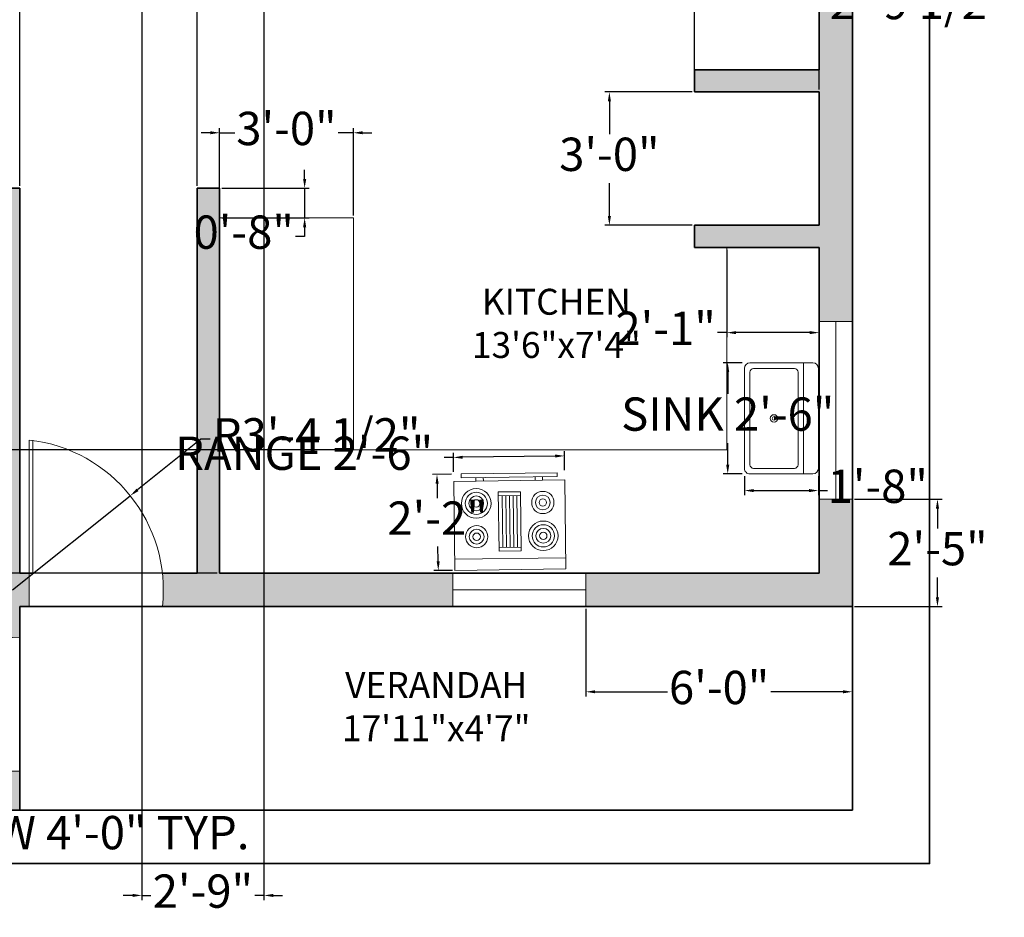
# Model space of a CAD drawing. Units: inches. Extents: x 1649 to 2193, y 1782 to 2280.
# Tile 2 of 3: x 1905 to 2171, y 1782 to 2024. Entities that reach past the tile are written whole.
import ezdxf

# ---------------------------------------------------------------- set-up
doc = ezdxf.new("R2010")
doc.units = ezdxf.units.IN
for name, color, linetype, lineweight in [('A-ANNO-DIMS', 2, 'Continuous', 18), ('A-ANNO-TTLB', 7, 'Continuous', 35), ('A-AREA-IDEN', 7, 'Continuous', 25), ('A-DOOR', 3, 'Continuous', 18), ('A-EQPM', 8, 'Continuous', 18), ('A-FLOR-CASE', 8, 'Continuous', 20), ('A-FLOR-FIXT', 9, 'Continuous', 18), ('A-GLAZ', 4, 'Continuous', 18), ('A-WALL', 7, 'Continuous', 35)]:
    doc.layers.add(name, color=color, linetype=linetype, lineweight=lineweight)
doc.layers.add('A-WALL-PATT', color=18, linetype='Continuous', lineweight=13, true_color=0x000000)
doc.styles.get("Standard").update_dxf_attribs({"font": 'arial.ttf'})
doc.dimstyles.new('ISO-25', dxfattribs={"dimtxt": 9, "dimasz": 2.5, "dimexe": 1.25, "dimexo": 0.625, "dimgap": 2, "dimtad": 0, "dimtih": 1, "dimtoh": 1, "dimdec": 1, "dimlunit": 4, "dimtxsty": 'Standard', "dimcen": 2.5, "dimadec": 0, "dimazin": 0, "dimtfac": 0.5, "dimtdec": 1, "dimtmove": 0, "dimatfit": 3, "dimfxl": 1, "dimarcsym": 0})

# ---------------------------------------------------------------- blocks, each defined once
blk = doc.blocks.new('Range-Oven - 30 in top')
for p, q in [((0, -3), (30, -3)), ((12, -6), (18, -6)), ((13, -20), (13, -6)), ((14, -6), (14, -20)), ((15, -20), (15, -6)), ((16, -6), (16, -20)), ((17, -20), (17, -6)), ((18, -20), (12, -20)), ((6, -24), (6, -25)), ((8, -25), (8, -24)), ((22, -25), (22, -24)), ((24, -24), (24, -25))]:
    blk.add_line(p, q)
for points in [[(0, -24), (0, 0), (30, 0), (30, -24)], [(12, -21), (12, -5), (18, -5), (18, -21)], [(2, -26), (2, -25), (28, -25), (28, -26)]]:
    blk.add_lwpolyline(points, close=True)
for centre, radius in [((6, -9), 4), ((6, -9), 3), ((6, -9), 2), ((24, -9), 3), ((24, -9), 2), ((6, -9), 1), ((24, -9), 1), ((6, -18), 3), ((24, -18), 4), ((24, -18), 3), ((6, -18), 2), ((6, -18), 1), ((24, -18), 2), ((24, -18), 1)]:
    blk.add_circle(centre, radius)
blk = doc.blocks.new('Sink-single - 30 in top')
blk.add_line((-15, -3.999996), (15, -3.999996))
for points in [[(-13.5, 0), (13.5, 0)], [(-15, -18.499996), (-15, -1.5)], [(15, -1.5), (15, -18.499996)], [(-13.5, -17.499996), (-13.5, -6.499996)], [(-12.5, -5.499996), (12.5, -5.499996)], [(13.5, -6.499996), (13.5, -17.499996)], [(12.5, -18.499996), (-12.5, -18.499996)], [(13.5, -19.999996), (-13.5, -19.999996)]]:
    blk.add_lwpolyline(points)
for radius in [1, 0.5]:
    blk.add_circle((0, -11.999996), radius)
for centre, radius, start, end in [((-13.5, -1.5), 1.5, 90, 180), ((13.5, -1.5), 1.5, 0, 90), ((-12.5, -6.499996), 1, 90, 180), ((12.5, -6.499996), 1, 0, 90), ((-13.5, -18.499996), 1.5, 180, 270), ((-12.5, -17.499996), 1, 180, 270), ((12.5, -17.499996), 1, 270, 0), ((13.5, -18.499996), 1.5, 270, 0)]:
    blk.add_arc(centre, radius, start, end)
blk = doc.blocks.new('DOOR-36IN')
for p, q in [((0, 6), (0, 42)), ((1, 6), (1, 42)), ((0, 6), (0, 0))]:
    blk.add_line(p, q)
blk.add_arc((-3, 3), 39.12, 355.6013, 85.6013)
blk = doc.blocks.new('WIN-48IN')
for p, q in [((0, 48), (9, 48)), ((4.5, 48), (4.5, 0)), ((0, 0), (9, 0))]:
    blk.add_line(p, q)
blk = doc.blocks.new('WIN-36IN')
for p, q in [((0, 9), (0, 0)), ((36, 9), (36, 0)), ((0, 4.5), (36, 4.5))]:
    blk.add_line(p, q)
blk = doc.blocks.new('*D23')
at = {"layer": 'A-ANNO-DIMS', "color": 0, "lineweight": -2, "transparency": 16777216}
for p, q in [((1803.13, 1810.03), (1803.13, 1802.2)), ((1851.13, 1810.03), (1851.13, 1802.2)), ((1805.63, 1803.45), (1848.63, 1803.45)), ((1851.13, 1803.45), (1853.63, 1803.45))]:
    blk.add_line(p, q, dxfattribs=at)
at = {"layer": 'A-ANNO-DIMS', "color": 0, "transparency": 16777216}
for points in [[(1805.63, 1803.87), (1805.63, 1803.04), (1803.13, 1803.45)], [(1848.63, 1803.87), (1848.63, 1803.04), (1851.13, 1803.45)]]:
    blk.add_solid(points, dxfattribs=at)
at = {"layer": 'Defpoints', "color": 0, "transparency": 16777216}
for p in [(1803.13, 1810.65), (1851.13, 1810.65), (1851.13, 1803.45)]:
    blk.add_point(p, dxfattribs=at)
at = {"layer": 'A-ANNO-DIMS', "color": 0, "transparency": 16777216, "insert": (1912.57, 1803.45), "char_height": 9, "attachment_point": 5}
blk.add_mtext('WINDOW 4\'-0" TYP.', dxfattribs=at)
blk = doc.blocks.new('*D29')
at = {"layer": 'A-ANNO-DIMS', "color": 0, "lineweight": -2, "transparency": 16777216}
for p, q in [((2022.33, 1905.95), (2019.83, 1905.92)), ((2022.39, 1902.08), (2022.32, 1907.2)), ((2049.83, 1906.32), (2024.83, 1905.98)), ((2052.38, 1902.48), (2052.31, 1907.61))]:
    blk.add_line(p, q, dxfattribs=at)
at = {"layer": 'A-ANNO-DIMS', "color": 0, "transparency": 16777216}
for points in [[(2024.83, 1906.4), (2024.84, 1905.57), (2022.33, 1905.95)], [(2049.82, 1906.74), (2049.84, 1905.91), (2052.33, 1906.36)]]:
    blk.add_solid(points, dxfattribs=at)
at = {"layer": 'Defpoints', "color": 0, "transparency": 16777216}
for p in [(2022.33, 1905.95), (2022.39, 1901.45), (2052.39, 1901.86)]:
    blk.add_point(p, dxfattribs=at)
at = {"layer": 'A-ANNO-DIMS', "color": 0, "transparency": 16777216, "insert": (1982, 1905.92), "char_height": 9, "attachment_point": 5}
blk.add_mtext('RANGE 2\'-6"', dxfattribs=at)
blk = doc.blocks.new('*D30')
at = {"layer": 'A-ANNO-DIMS', "color": 0, "lineweight": -2, "transparency": 16777216}
for p, q in [((2021.77, 1901.44), (2016.64, 1901.37)), ((2017.93, 1898.89), (2017.98, 1894.91)), ((2018.21, 1877.89), (2018.16, 1881.87)), ((2022.12, 1875.44), (2017, 1875.38))]:
    blk.add_line(p, q, dxfattribs=at)
at = {"layer": 'A-ANNO-DIMS', "color": 0, "transparency": 16777216}
for points in [[(2018.34, 1898.9), (2017.51, 1898.88), (2017.89, 1901.39)], [(2018.63, 1877.9), (2017.8, 1877.89), (2018.25, 1875.39)]]:
    blk.add_solid(points, dxfattribs=at)
at = {"layer": 'Defpoints', "color": 0, "transparency": 16777216}
for p in [(2022.39, 1901.45), (2018.25, 1875.39), (2022.75, 1875.45)]:
    blk.add_point(p, dxfattribs=at)
at = {"layer": 'A-ANNO-DIMS', "color": 0, "transparency": 16777216, "insert": (2018.07, 1888.39), "char_height": 9, "attachment_point": 5}
blk.add_mtext('2\'-2"', dxfattribs=at)
blk = doc.blocks.new('*D31')
at = {"layer": 'A-ANNO-DIMS', "color": 0, "lineweight": -2, "transparency": 16777216}
for p, q in [((2100.33, 1931.49), (2095.21, 1931.49)), ((2096.46, 1928.99), (2096.46, 1923.15)), ((2096.46, 1903.99), (2096.46, 1909.84)), ((2100.33, 1901.49), (2095.21, 1901.49))]:
    blk.add_line(p, q, dxfattribs=at)
at = {"layer": 'A-ANNO-DIMS', "color": 0, "transparency": 16777216}
for points in [[(2096.04, 1928.99), (2096.87, 1928.99), (2096.46, 1931.49)], [(2096.04, 1903.99), (2096.87, 1903.99), (2096.46, 1901.49)]]:
    blk.add_solid(points, dxfattribs=at)
at = {"layer": 'Defpoints', "color": 0, "transparency": 16777216}
for p in [(2100.96, 1931.49), (2096.46, 1901.49), (2100.96, 1901.49)]:
    blk.add_point(p, dxfattribs=at)
at = {"layer": 'A-ANNO-DIMS', "color": 0, "transparency": 16777216, "insert": (2096.46, 1916.49), "char_height": 9, "attachment_point": 5}
blk.add_mtext('SINK 2\'-6"', dxfattribs=at)
blk = doc.blocks.new('*D32')
at = {"layer": 'A-ANNO-DIMS', "color": 0, "lineweight": -2, "transparency": 16777216}
for p, q in [((2100.96, 1900.87), (2100.96, 1895.74)), ((2120.96, 1900.87), (2120.96, 1895.74)), ((2103.46, 1896.99), (2118.46, 1896.99)), ((2120.96, 1896.99), (2123.46, 1896.99))]:
    blk.add_line(p, q, dxfattribs=at)
at = {"layer": 'A-ANNO-DIMS', "color": 0, "transparency": 16777216}
for points in [[(2103.46, 1897.41), (2103.46, 1896.58), (2100.96, 1896.99)], [(2118.46, 1897.41), (2118.46, 1896.58), (2120.96, 1896.99)]]:
    blk.add_solid(points, dxfattribs=at)
at = {"layer": 'Defpoints', "color": 0, "transparency": 16777216}
for p in [(2100.96, 1901.49), (2120.96, 1901.49), (2120.96, 1896.99)]:
    blk.add_point(p, dxfattribs=at)
at = {"layer": 'A-ANNO-DIMS', "color": 0, "transparency": 16777216, "insert": (2137, 1896.99), "char_height": 9, "attachment_point": 5}
blk.add_mtext('1\'-8"', dxfattribs=at)
blk = doc.blocks.new('*D36')
at = {"layer": 'A-ANNO-DIMS', "color": 0, "lineweight": -2, "transparency": 16777216}
for p, q in [((1905.13, 1979.28), (1905.13, 2266.9)), ((1953.13, 1979.28), (1953.13, 2266.9)), ((1907.63, 2265.65), (1914.99, 2265.65)), ((1950.63, 2265.65), (1943.27, 2265.65))]:
    blk.add_line(p, q, dxfattribs=at)
at = {"layer": 'A-ANNO-DIMS', "color": 0, "transparency": 16777216}
for points in [[(1907.63, 2266.07), (1907.63, 2265.24), (1905.13, 2265.65)], [(1950.63, 2266.07), (1950.63, 2265.24), (1953.13, 2265.65)]]:
    blk.add_solid(points, dxfattribs=at)
at = {"layer": 'Defpoints', "color": 0, "transparency": 16777216}
for p in [(1953.13, 2265.65), (1905.13, 1978.65), (1953.13, 1978.65)]:
    blk.add_point(p, dxfattribs=at)
at = {"layer": 'A-ANNO-DIMS', "color": 0, "transparency": 16777216, "insert": (1929.13, 2265.65), "char_height": 9, "attachment_point": 5}
blk.add_mtext('4\'-0"', dxfattribs=at)
blk = doc.blocks.new('*D41')
at = {"layer": 'A-ANNO-DIMS', "color": 0, "lineweight": -2, "transparency": 16777216}
for p, q in [((2058.13, 1865.03), (2058.13, 1841.4)), ((2130.13, 1865.03), (2130.13, 1841.4)), ((2060.63, 1842.65), (2080.14, 1842.65)), ((2127.63, 1842.65), (2108.12, 1842.65))]:
    blk.add_line(p, q, dxfattribs=at)
at = {"layer": 'A-ANNO-DIMS', "color": 0, "transparency": 16777216}
for points in [[(2060.63, 1843.07), (2060.63, 1842.24), (2058.13, 1842.65)], [(2127.63, 1843.07), (2127.63, 1842.24), (2130.13, 1842.65)]]:
    blk.add_solid(points, dxfattribs=at)
at = {"layer": 'Defpoints', "color": 0, "transparency": 16777216}
for p in [(2058.13, 1865.65), (2130.13, 1865.65), (2058.13, 1842.65)]:
    blk.add_point(p, dxfattribs=at)
at = {"layer": 'A-ANNO-DIMS', "color": 0, "transparency": 16777216, "insert": (2094.13, 1842.65), "char_height": 9, "attachment_point": 5}
blk.add_mtext('6\'-0"', dxfattribs=at)
blk = doc.blocks.new('*D42')
at = {"layer": 'A-ANNO-DIMS', "color": 0, "lineweight": -2, "transparency": 16777216}
for p, q in [((2130.75, 1894.65), (2154.38, 1894.65)), ((2153.13, 1892.15), (2153.13, 1886.75)), ((2153.13, 1868.15), (2153.13, 1873.56)), ((2130.75, 1865.65), (2154.38, 1865.65))]:
    blk.add_line(p, q, dxfattribs=at)
at = {"layer": 'A-ANNO-DIMS', "color": 0, "transparency": 16777216}
for points in [[(2152.71, 1892.15), (2153.55, 1892.15), (2153.13, 1894.65)], [(2152.71, 1868.15), (2153.55, 1868.15), (2153.13, 1865.65)]]:
    blk.add_solid(points, dxfattribs=at)
at = {"layer": 'Defpoints', "color": 0, "transparency": 16777216}
for p in [(2130.13, 1894.65), (2153.13, 1894.65), (2130.13, 1865.65)]:
    blk.add_point(p, dxfattribs=at)
at = {"layer": 'A-ANNO-DIMS', "color": 0, "transparency": 16777216, "insert": (2153.13, 1880.15), "char_height": 9, "attachment_point": 5}
blk.add_mtext('2\'-5"', dxfattribs=at)
blk = doc.blocks.new('*D51')
at = {"layer": 'A-ANNO-DIMS', "color": 0, "lineweight": -2, "transparency": 16777216}
for p, q in [((1938.13, 2212.02), (1938.13, 1786.4)), ((1971.13, 2201.52), (1971.13, 1786.4)), ((1935.63, 1787.65), (1933.13, 1787.65)), ((1938.13, 1787.65), (1940.59, 1787.65)), ((1971.13, 1787.65), (1968.67, 1787.65)), ((1973.63, 1787.65), (1976.13, 1787.65))]:
    blk.add_line(p, q, dxfattribs=at)
at = {"layer": 'A-ANNO-DIMS', "color": 0, "transparency": 16777216}
for points in [[(1935.63, 1788.07), (1935.63, 1787.24), (1938.13, 1787.65)], [(1973.63, 1788.07), (1973.63, 1787.24), (1971.13, 1787.65)]]:
    blk.add_solid(points, dxfattribs=at)
at = {"layer": 'Defpoints', "color": 0, "transparency": 16777216}
for p in [(1938.13, 2212.65), (1971.13, 2202.15), (1971.13, 1787.65)]:
    blk.add_point(p, dxfattribs=at)
at = {"layer": 'A-ANNO-DIMS', "color": 0, "transparency": 16777216, "insert": (1954.63, 1787.65), "char_height": 9, "attachment_point": 5}
blk.add_mtext('2\'-9"', dxfattribs=at)
blk = doc.blocks.new('*D54')
at = {"layer": 'A-ANNO-DIMS', "color": 0, "lineweight": -2, "transparency": 16777216}
for p, q in [((2087.48, 2005.28), (2087.48, 2028.9)), ((2089.98, 2027.65), (2118.63, 2027.65)), ((2121.13, 2005.28), (2121.13, 2028.9)), ((2121.13, 2027.65), (2123.63, 2027.65))]:
    blk.add_line(p, q, dxfattribs=at)
at = {"layer": 'A-ANNO-DIMS', "color": 0, "transparency": 16777216}
for points in [[(2089.98, 2028.07), (2089.98, 2027.24), (2087.48, 2027.65)], [(2118.63, 2028.07), (2118.63, 2027.24), (2121.13, 2027.65)]]:
    blk.add_solid(points, dxfattribs=at)
at = {"layer": 'Defpoints', "color": 0, "transparency": 16777216}
for p in [(2121.13, 2027.65), (2087.48, 2004.65), (2121.13, 2004.65)]:
    blk.add_point(p, dxfattribs=at)
at = {"layer": 'A-ANNO-DIMS', "color": 0, "transparency": 16777216, "insert": (2148.15, 2027.65), "char_height": 9, "attachment_point": 5}
blk.add_mtext('2\'-9 1/2"', dxfattribs=at)
blk = doc.blocks.new('*D55')
at = {"layer": 'A-ANNO-DIMS', "color": 0, "lineweight": -2, "transparency": 16777216}
for p, q in [((2086.85, 2004.65), (2063.23, 2004.65)), ((2064.48, 2002.15), (2064.48, 1993.25)), ((2064.48, 1971.15), (2064.48, 1980.05)), ((2086.85, 1968.65), (2063.23, 1968.65))]:
    blk.add_line(p, q, dxfattribs=at)
at = {"layer": 'A-ANNO-DIMS', "color": 0, "transparency": 16777216}
for points in [[(2064.06, 2002.15), (2064.89, 2002.15), (2064.48, 2004.65)], [(2064.06, 1971.15), (2064.89, 1971.15), (2064.48, 1968.65)]]:
    blk.add_solid(points, dxfattribs=at)
at = {"layer": 'Defpoints', "color": 0, "transparency": 16777216}
for p in [(2064.48, 2004.65), (2087.48, 2004.65), (2087.48, 1968.65)]:
    blk.add_point(p, dxfattribs=at)
at = {"layer": 'A-ANNO-DIMS', "color": 0, "transparency": 16777216, "insert": (2064.48, 1986.65), "char_height": 9, "attachment_point": 5}
blk.add_mtext('3\'-0"', dxfattribs=at)
blk = doc.blocks.new('*D56')
at = {"layer": 'A-ANNO-DIMS', "color": 0, "lineweight": -2, "transparency": 16777216}
for p, q in [((2096.22, 1962.03), (2096.22, 1938.4)), ((2121.13, 1962.03), (2121.13, 1938.4)), ((2096.22, 1939.65), (2093.72, 1939.65)), ((2118.63, 1939.65), (2098.72, 1939.65))]:
    blk.add_line(p, q, dxfattribs=at)
at = {"layer": 'A-ANNO-DIMS', "color": 0, "transparency": 16777216}
for points in [[(2098.72, 1940.07), (2098.72, 1939.24), (2096.22, 1939.65)], [(2118.63, 1940.07), (2118.63, 1939.24), (2121.13, 1939.65)]]:
    blk.add_solid(points, dxfattribs=at)
at = {"layer": 'Defpoints', "color": 0, "transparency": 16777216}
for p in [(2096.22, 1962.65), (2121.13, 1962.65), (2096.22, 1939.65)]:
    blk.add_point(p, dxfattribs=at)
at = {"layer": 'A-ANNO-DIMS', "color": 0, "transparency": 16777216, "insert": (2079.68, 1939.65), "char_height": 9, "attachment_point": 5}
blk.add_mtext('2\'-1"', dxfattribs=at)
blk = doc.blocks.new('*D57')
at = {"layer": 'A-ANNO-DIMS', "color": 0, "lineweight": -2, "transparency": 16777216}
for p, q in [((1956.63, 1993.63), (1954.13, 1993.63)), ((1959.13, 1971.26), (1959.13, 1994.88)), ((1959.13, 1993.63), (1963.25, 1993.63)), ((1995.3, 1993.63), (1991.17, 1993.63)), ((1995.3, 1971.26), (1995.3, 1994.88)), ((1997.8, 1993.63), (2000.3, 1993.63))]:
    blk.add_line(p, q, dxfattribs=at)
at = {"layer": 'A-ANNO-DIMS', "color": 0, "transparency": 16777216}
for points in [[(1956.63, 1994.05), (1956.63, 1993.22), (1959.13, 1993.63)], [(1997.8, 1994.05), (1997.8, 1993.22), (1995.3, 1993.63)]]:
    blk.add_solid(points, dxfattribs=at)
at = {"layer": 'Defpoints', "color": 0, "transparency": 16777216}
for p in [(1995.3, 1993.63), (1959.13, 1970.63), (1995.3, 1970.63)]:
    blk.add_point(p, dxfattribs=at)
at = {"layer": 'A-ANNO-DIMS', "color": 0, "transparency": 16777216, "insert": (1977.21, 1993.63), "char_height": 9, "attachment_point": 5}
blk.add_mtext('3\'-0"', dxfattribs=at)
blk = doc.blocks.new('*D58')
at = {"layer": 'A-ANNO-DIMS', "color": 0, "lineweight": -2, "transparency": 16777216}
for p, q in [((1994.67, 1908.03), (1671.31, 1908.03)), ((1672.56, 1905.53), (1672.56, 1898)), ((1672.56, 1877.15), (1672.56, 1884.69)), ((1958.5, 1874.65), (1671.31, 1874.65))]:
    blk.add_line(p, q, dxfattribs=at)
at = {"layer": 'A-ANNO-DIMS', "color": 0, "transparency": 16777216}
for points in [[(1672.15, 1905.53), (1672.98, 1905.53), (1672.56, 1908.03)], [(1672.15, 1877.15), (1672.98, 1877.15), (1672.56, 1874.65)]]:
    blk.add_solid(points, dxfattribs=at)
at = {"layer": 'Defpoints', "color": 0, "transparency": 16777216}
for p in [(1995.3, 1908.03), (1672.56, 1874.65), (1959.13, 1874.65)]:
    blk.add_point(p, dxfattribs=at)
at = {"layer": 'A-ANNO-DIMS', "color": 0, "transparency": 16777216, "insert": (1672.56, 1891.34), "char_height": 9, "attachment_point": 5}
blk.add_mtext('2\'-9 1/2"', dxfattribs=at)
blk = doc.blocks.new('*D59')
at = {"layer": 'A-ANNO-DIMS', "color": 0, "lineweight": -2, "transparency": 16777216}
for p, q in [((1982.13, 1981.15), (1982.13, 1983.65)), ((1959.75, 1978.65), (1983.38, 1978.65)), ((1982.13, 1978.65), (1982.13, 1970.63)), ((1959.75, 1970.63), (1983.38, 1970.63)), ((1982.13, 1968.13), (1982.13, 1965.63)), ((1982.13, 1965.63), (1979.63, 1965.63))]:
    blk.add_line(p, q, dxfattribs=at)
at = {"layer": 'A-ANNO-DIMS', "color": 0, "transparency": 16777216}
for points in [[(1981.71, 1981.15), (1982.55, 1981.15), (1982.13, 1978.65)], [(1981.71, 1968.13), (1982.55, 1968.13), (1982.13, 1970.63)]]:
    blk.add_solid(points, dxfattribs=at)
at = {"layer": 'Defpoints', "color": 0, "transparency": 16777216}
for p in [(1959.13, 1978.65), (1959.13, 1970.63), (1982.13, 1970.63)]:
    blk.add_point(p, dxfattribs=at)
at = {"layer": 'A-ANNO-DIMS', "color": 0, "transparency": 16777216, "insert": (1965.67, 1965.63), "char_height": 9, "attachment_point": 5}
blk.add_mtext('0\'-8"', dxfattribs=at)
blk = doc.blocks.new('*D61')
at = {"layer": 'A-ANNO-DIMS', "color": 0, "lineweight": -2, "transparency": 16777216}
for p, q in [((1954.1, 1910.88), (1936.96, 1897.17)), ((1956.6, 1910.88), (1954.1, 1910.88)), ((1903.19, 1870.15), (1935.01, 1895.61))]:
    blk.add_line(p, q, dxfattribs=at)
at = {"layer": 'A-ANNO-DIMS', "color": 0, "transparency": 16777216}
blk.add_solid([(1936.7, 1897.5), (1937.22, 1896.84), (1935.01, 1895.61)], dxfattribs=at)
at = {"layer": 'Defpoints', "color": 0, "transparency": 16777216}
for p in [(1935.01, 1895.61), (1903.19, 1870.15)]:
    blk.add_point(p, dxfattribs=at)
at = {"layer": 'A-ANNO-DIMS', "color": 0, "transparency": 16777216, "insert": (1985.35, 1910.88), "char_height": 9, "attachment_point": 5}
blk.add_mtext('R3\'-4 1/2"', dxfattribs=at)

msp = doc.modelspace()

# ---------------------------------------------------------------- hatches: boundary and pattern name
at = {"layer": 'A-WALL-PATT'}
h = msp.add_hatch(color=256, dxfattribs=at)
h.dxf.hatch_style = 1
h.paths.add_polyline_path([(1926.13, 2242.65), (1746.13, 2242.65), (1746.13, 2203.65), (1755.13, 2203.65), (1755.13, 2233.65), (1899.13, 2233.65), (1899.13, 2113.65), (1897.63, 2113.65), (1897.63, 2107.65), (1899.13, 2107.65), (1907.03, 2107.65), (1907.03, 2113.65), (1905.13, 2113.65), (1905.13, 2233.65), (1926.13, 2233.65)])
h.paths.add_polyline_path([(2130.13, 2242.65), (1950.13, 2242.65), (1950.13, 2233.65), (1971.13, 2233.65), (1971.13, 2113.65), (1937.03, 2113.65, -0.045361), (1937.03, 2107.65), (1978.81, 2107.65), (1978.81, 2113.65), (1977.13, 2113.65), (1977.13, 2233.65), (2121.13, 2233.65), (2121.13, 2203.65), (2130.13, 2203.65)])
h.paths.add_polyline_path([(2130.13, 2143.65), (2121.13, 2143.65), (2121.13, 2113.65), (2014.81, 2113.65, -0.038405), (2014.81, 2107.65), (2121.13, 2107.65), (2121.13, 2089.15), (2130.13, 2089.15)])
h.paths.add_polyline_path([(1824.23, 2113.65), (1755.13, 2113.65), (1755.13, 2143.65), (1746.13, 2143.65), (1746.13, 2093.65), (1755.13, 2093.65), (1755.13, 2107.65), (1824.23, 2107.65, -0.045361)])
h.paths.add_polyline_path([(1862.13, 2055.65), (1862.13, 2107.65), (1863.33, 2107.65, -0.038218), (1863.33, 2113.65), (1854.23, 2113.65), (1854.23, 2107.65), (1856.13, 2107.65), (1856.13, 2055.65), (1755.13, 2055.65), (1755.13, 2069.65), (1746.13, 2069.65), (1746.13, 2032.15), (1755.13, 2032.15), (1755.13, 2049.65), (1862.13, 2049.65)])
h.paths.add_polyline_path([(2130.13, 2029.15), (2121.13, 2029.15), (2121.13, 2010.65), (2087.48, 2010.65), (2087.48, 2004.65), (2121.13, 2004.65), (2121.13, 1968.65), (2087.48, 1968.65), (2087.48, 1962.65), (2121.13, 1962.65), (2121.13, 1942.65), (2130.13, 1942.65)])
h.paths.add_polyline_path([(2022.13, 1874.65), (1959.13, 1874.65), (1959.13, 1978.65), (1953.13, 1978.65), (1953.13, 1874.65), (1943.69, 1874.65, -0.055385), (1943.69, 1865.65), (2022.13, 1865.65)])
h.paths.add_polyline_path([(2130.13, 1894.65), (2121.13, 1894.65), (2121.13, 1874.65), (2058.13, 1874.65), (2058.13, 1865.65), (2121.13, 1865.65), (2130.13, 1865.65)])
h.paths.add_polyline_path([(1755.13, 1972.65), (1859.98, 1972.65, -0.038405), (1859.98, 1978.65), (1755.13, 1978.65), (1755.13, 1996.15), (1746.13, 1996.15), (1746.13, 1920.15), (1755.13, 1920.15)])
h.paths.add_polyline_path([(1803.13, 1819.65), (1755.13, 1819.65), (1755.13, 1872.15), (1746.13, 1872.15), (1746.13, 1810.65), (1803.13, 1810.65)])
h.paths.add_polyline_path([(1905.13, 1819.65), (1905.13, 1821.19), (1899.13, 1821.19), (1899.13, 1819.65), (1851.13, 1819.65), (1851.13, 1810.65), (1905.13, 1810.65)])
h.paths.add_polyline_path([(1907.69, 1874.65), (1905.13, 1874.65), (1905.13, 1972.65), (1905.13, 1978.65), (1895.98, 1978.65), (1895.98, 1972.65), (1899.13, 1972.65), (1899.13, 1857.19, -0.038405), (1905.13, 1857.19), (1905.13, 1865.65), (1907.69, 1865.65)])

# ---------------------------------------------------------------- linework, layer by layer
at = {"layer": 'A-ANNO-TTLB'}
msp.add_lwpolyline([(1708.93, 2280.02), (2150.99, 2280.02), (2150.99, 1796.25), (1708.93, 1796.25)], close=True, dxfattribs=at)
at = {"layer": 'A-DOOR'}
for p, q in [((1907.69, 1874.65), (1907.69, 1910.65)), ((1908.69, 1874.65), (1908.69, 1910.65)), ((1907.69, 1874.65), (1907.69, 1865.65))]:
    msp.add_line(p, q, dxfattribs=at)
msp.add_arc((1903.19, 1870.15), 40.75, 353.6598, 83.6598, dxfattribs=at)
at = {"layer": 'A-FLOR-CASE'}
for p, q in [((1995.3, 1970.63), (1959.13, 1970.63)), ((1995.3, 1908.03), (1995.3, 1970.63)), ((2096.22, 1962.65), (2096.22, 1908.03)), ((2096.22, 1908.03), (1995.3, 1908.03))]:
    msp.add_line(p, q, dxfattribs=at)
at = {"layer": 'A-WALL'}
for p, q in [((2130.13, 2242.65), (2130.13, 1810.65)), ((2121.13, 2107.65), (2121.13, 2010.65)), ((2121.13, 2010.65), (2087.48, 2010.65)), ((2087.48, 2004.65), (2087.48, 2010.65)), ((2121.13, 2004.65), (2087.48, 2004.65)), ((2121.13, 1968.65), (2121.13, 2004.65)), ((2121.13, 2004.65), (2121.13, 1968.65)), ((1905.13, 1978.65), (1755.13, 1978.65)), ((1905.13, 1972.65), (1905.13, 1978.65)), ((1953.13, 1978.65), (1953.13, 1874.65)), ((1953.13, 1978.65), (1959.13, 1978.65)), ((1959.13, 1978.65), (1959.13, 1874.65)), ((1905.13, 1874.65), (1905.13, 1972.65)), ((2121.13, 1968.65), (2087.48, 1968.65)), ((2087.48, 1968.65), (2087.48, 1962.65)), ((2121.13, 1962.65), (2087.48, 1962.65)), ((2121.13, 1962.65), (2121.13, 1874.65)), ((1908.69, 1874.65), (1905.13, 1874.65)), ((1953.13, 1874.65), (1943.69, 1874.65)), ((2121.13, 1874.65), (1959.13, 1874.65)), ((1905.13, 1819.65), (1905.13, 1865.65)), ((2121.13, 1865.65), (1905.13, 1865.65)), ((2121.13, 1865.65), (2130.13, 1865.65)), ((1905.13, 1819.65), (1905.13, 1810.65)), ((2130.13, 1810.65), (1746.13, 1810.65))]:
    msp.add_line(p, q, dxfattribs=at)

# ---------------------------------------------------------------- block references
at = {"layer": 'A-DOOR', "rotation": 89.99999999999905}
msp.add_blockref('DOOR-36IN', (1905.13, 1821.19), dxfattribs=at)
at = {"layer": 'A-EQPM', "rotation": 180.7771274632593}
msp.add_blockref('Range-Oven - 30 in top', (2052.74, 1875.86), dxfattribs=at)
at = {"layer": 'A-FLOR-FIXT', "rotation": 270}
msp.add_blockref('Sink-single - 30 in top', (2120.96, 1916.49), dxfattribs=at)
at = {"layer": 'A-GLAZ'}
for name, p in [('WIN-48IN', (2121.13, 1894.65)), ('WIN-36IN', (2022.13, 1865.65))]:
    msp.add_blockref(name, p, dxfattribs=at)

# ---------------------------------------------------------------- texts
at = {"layer": 'A-AREA-IDEN', "char_height": 7, "attachment_point": 1}
for s, width, insert in [('\\pxqc;{\\fArial|b1|i0|c0|p34;KITCHEN\\P13\'6"x7\'4"}', 92.1713, (2004.05, 1951.49)), ('\\pxqc;{\\fArial|b1|i0|c0|p34;VERANDAH\\P17\'11"x4\'7"}', 107.1133, (1964.13, 1847.98))]:
    msp.add_mtext_dynamic_manual_height_columns(s, width=width, gutter_width=12.5, heights=[0], dxfattribs=dict(at, insert=insert))

# ---------------------------------------------------------------- dimensions: what is measured, and where the dimension line sits
at = {"layer": 'A-ANNO-DIMS'}
for base, p1, p2, picture, middle in [((1953.13, 2265.65), (1905.13, 1978.65), (1953.13, 1978.65), '*D36', (1929.13, 2265.65)), ((1971.13, 1787.65), (1938.13, 2212.65), (1971.13, 2202.15), '*D51', (1954.63, 1787.65)), ((2121.1289, 2027.6524), (2087.4781, 2004.6524), (2121.1289, 2004.6524), '*D54', (2148.1535, 2027.6524)), ((1995.3, 1993.63), (1959.13, 1970.63), (1995.3, 1970.63), '*D57', (1977.21, 1993.63)), ((2120.96, 1896.99), (2100.96, 1901.49), (2120.96, 1901.49), '*D32', (2137, 1896.99))]:
    dim = msp.add_linear_dim(base=base, p1=p1, p2=p2, dimstyle='ISO-25', override={"dimdec": 1, "dimlfac": 1, "dimrnd": 0, "dimzin": 1, "dimdsep": 46, "dimlunit": 4, "dimfrac": 2}, dxfattribs=at)
    dim.commit()
    dim.dimension.update_dxf_attribs({"geometry": picture, "text_midpoint": middle})
for base, p1, p2, angle, picture, middle in [((2064.48, 2004.65), (2087.48, 1968.65), (2087.48, 2004.65), 90, '*D55', (2064.48, 1986.65)), ((1982.13, 1970.63), (1959.13, 1978.65), (1959.13, 1970.63), 270, '*D59', (1965.67, 1965.63)), ((2096.22, 1939.65), (2121.13, 1962.65), (2096.22, 1962.65), 180, '*D56', (2079.68, 1939.65)), ((1672.56, 1874.65), (1995.3, 1908.03), (1959.13, 1874.65), 90, '*D58', (1672.56, 1891.34)), ((2018.25, 1875.39), (2022.39, 1901.45), (2022.75, 1875.45), 270.7771, '*D30', (2018.07, 1888.39)), ((2153.13, 1894.65), (2130.13, 1865.65), (2130.13, 1894.65), 90, '*D42', (2153.13, 1880.15)), ((2058.13, 1842.65), (2130.13, 1865.65), (2058.13, 1865.65), 180, '*D41', (2094.13, 1842.65))]:
    dim = msp.add_linear_dim(base=base, p1=p1, p2=p2, angle=angle, dimstyle='ISO-25', override={"dimdec": 1, "dimlfac": 1, "dimrnd": 0, "dimzin": 1, "dimdsep": 46, "dimlunit": 4, "dimfrac": 2}, dxfattribs=at)
    dim.commit()
    dim.dimension.update_dxf_attribs({"geometry": picture, "text_midpoint": middle})
for base, p1, p2, angle, text, picture, middle in [((2096.46, 1901.49), (2100.96, 1931.49), (2100.96, 1901.49), 270, 'SINK <>', '*D31', (2096.46, 1916.49)), ((2022.33, 1905.95), (2052.39, 1901.86), (2022.39, 1901.45), 180.7771, 'RANGE <>', '*D29', (1982, 1905.92))]:
    dim = msp.add_linear_dim(base=base, p1=p1, p2=p2, angle=angle, text=text, dimstyle='ISO-25', override={"dimdec": 1, "dimlfac": 1, "dimrnd": 0, "dimzin": 1, "dimdsep": 46, "dimlunit": 4, "dimfrac": 2}, dxfattribs=at)
    dim.commit()
    dim.dimension.update_dxf_attribs({"geometry": picture, "text_midpoint": middle})
dim = msp.add_radius_dim(center=(1903.1856, 1870.1524), mpoint=(1935.0054, 1895.6083), dimstyle='ISO-25', override={"dimdec": 1, "dimlfac": 1, "dimrnd": 0, "dimzin": 1, "dimdsep": 46, "dimlunit": 4, "dimfrac": 2}, dxfattribs=at)
dim.commit()
dim.dimension.update_dxf_attribs({"geometry": '*D61', "text_midpoint": (1985.3516, 1910.8818), "dimtype": 164})
dim = msp.add_linear_dim(base=(1851.13, 1803.45), p1=(1803.13, 1810.65), p2=(1851.13, 1810.65), text='WINDOW <> TYP.', dimstyle='ISO-25', override={"dimdec": 1, "dimlfac": 1, "dimrnd": 0, "dimzin": 1, "dimdsep": 46, "dimlunit": 4, "dimfrac": 2}, dxfattribs=at)
dim.commit()
dim.dimension.update_dxf_attribs({"geometry": '*D23', "text_midpoint": (1912.57, 1803.45)})

doc.saveas('drawing.dxf')
